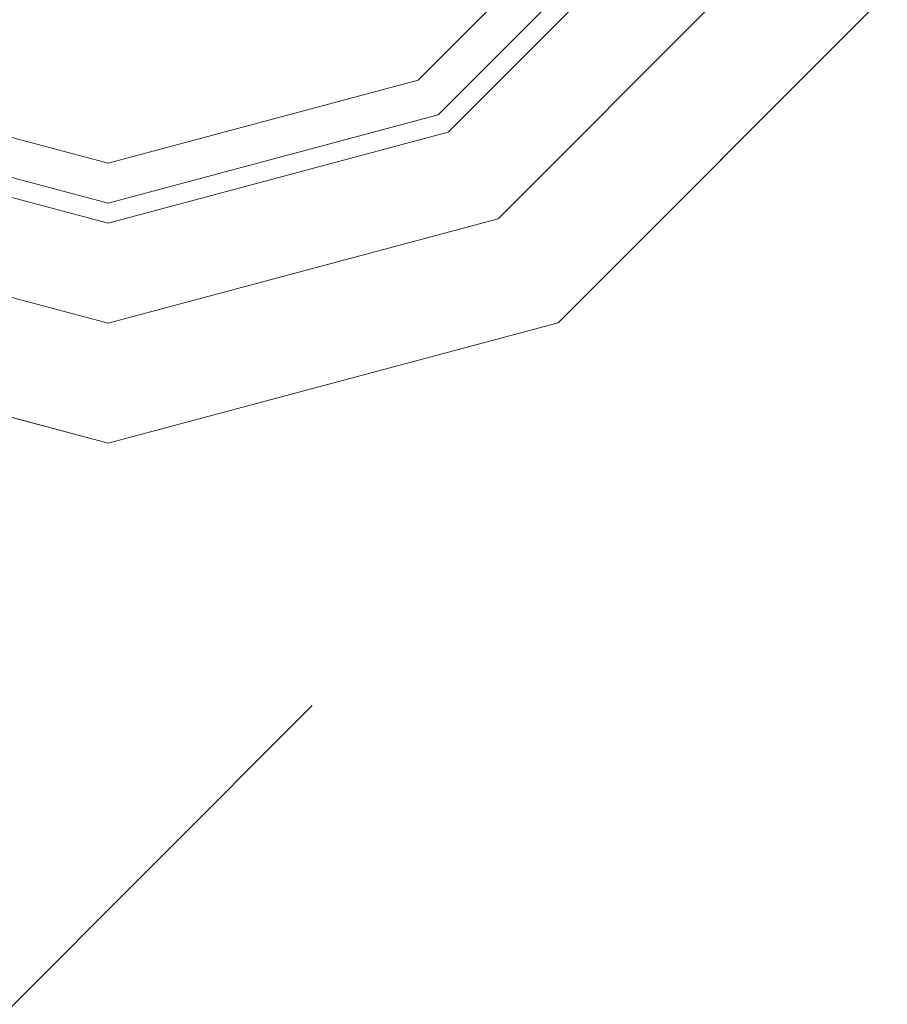
# Model space of a CAD drawing. Units: inches. Extents: x 375 to 1122, y 27 to 1069.
# Tile 53 of 155: x 725.537 to 730.88, y 308.183 to 314.242. Entities that reach past the tile are written whole.
import ezdxf

# ---------------------------------------------------------------- set-up
doc = ezdxf.new("R2010")
doc.units = ezdxf.units.IN
doc.layers.add('Furniture', color=30, linetype='Continuous', lineweight=18)

# ---------------------------------------------------------------- blocks, each defined once
blk = doc.blocks.new('A$C403C54AD')
blk.add_line((0.90685, 1.05977, -0.0006), (1.01943, 0.94723, -0.0006))
at = {"linetype": 'ByBlock'}
for points, invisible_edges in [([(0.81861, 1.08071, -0.03355), (0.84793, 1.09765, -0.02431), (0.79723, 1.14835, -0.02431), (0.7803, 1.11902, -0.03355)], 5), ([(0.84793, 1.09765, -0.0197), (0.83194, 1.08841, -0.0197), (0.78799, 1.13235, -0.0197), (0.79723, 1.14835, -0.0197)], 5), ([(0.83194, 1.08841, -0.0197), (0.81594, 1.07918, -0.02585), (0.77876, 1.11636, -0.02585), (0.78799, 1.13235, -0.0197)], 5), ([(0.81061, 1.0761, -0.04278), (0.81861, 1.08071, -0.03355), (0.7803, 1.11902, -0.03355), (0.77568, 1.11103, -0.04278)], 1), ([(0.81594, 1.07918, -0.02585), (0.72796, 1.02838, -0.02585), (0.72796, 1.02838, -0.02585), (0.77876, 1.11636, -0.02585)], 5), ([(0.83263, 1.02838, -0.03355), (0.86649, 1.02838, -0.02431), (0.84793, 1.09765, -0.02431), (0.81861, 1.08071, -0.03355)], 5), ([(0.86649, 1.02838, -0.0197), (0.84802, 1.02838, -0.0197), (0.83194, 1.08841, -0.0197), (0.84793, 1.09765, -0.0197)], 5), ([(0.84802, 1.02838, -0.0197), (0.82955, 1.02838, -0.02585), (0.81594, 1.07918, -0.02585), (0.83194, 1.08841, -0.0197)], 5), ([(0.82339, 1.02838, -0.04278), (0.83263, 1.02838, -0.03355), (0.81861, 1.08071, -0.03355), (0.81061, 1.0761, -0.04278)], 5), ([(0.82955, 1.02838, -0.02585), (0.72796, 1.02838, -0.02585), (0.72796, 1.02838, -0.02585), (0.81594, 1.07918, -0.02585)], 5), ([(0.81594, 0.97759, -0.02585), (0.72796, 1.02838, -0.02585), (0.72796, 1.02838, -0.02585), (0.82955, 1.02838, -0.02585)], 5), ([(0.77876, 0.94041, -0.02585), (0.72796, 1.02838, -0.02585), (0.72796, 1.02838, -0.02585), (0.81594, 0.97759, -0.02585)], 5), ([(0.81061, 0.98067, -0.04278), (0.81861, 0.97605, -0.03355), (0.83263, 1.02838, -0.03355), (0.82339, 1.02838, -0.04278)], 5), ([(0.83194, 0.96835, -0.0197), (0.81594, 0.97759, -0.02585), (0.82955, 1.02838, -0.02585), (0.84802, 1.02838, -0.0197)], 5), ([(0.81861, 0.97605, -0.03355), (0.84793, 0.95912, -0.02431), (0.86649, 1.02838, -0.02431), (0.83263, 1.02838, -0.03355)], 5), ([(0.84793, 0.95912, -0.0197), (0.83194, 0.96835, -0.0197), (0.84802, 1.02838, -0.0197), (0.86649, 1.02838, -0.0197)], 5)]:
    blk.add_3dface(points, dxfattribs=dict(at, invisible_edges=invisible_edges))
for points in [[(0.84793, 1.09765, -0.02431), (0.84793, 1.09765, -0.0197), (0.79723, 1.14835, -0.0197), (0.79723, 1.14835, -0.02431)], [(0.86649, 1.02838, -0.02431), (0.86649, 1.02838, -0.0197), (0.84793, 1.09765, -0.0197), (0.84793, 1.09765, -0.02431)], [(0.84793, 0.95912, -0.02431), (0.84793, 0.95912, -0.0197), (0.86649, 1.02838, -0.0197), (0.86649, 1.02838, -0.02431)]]:
    blk.add_3dface(points, dxfattribs=at)

msp = doc.modelspace()

# ---------------------------------------------------------------- block references
at = {"layer": 'Furniture', "xscale": 39.9918517141215, "yscale": 39.9918517141215, "zscale": 39.9918517141215, "rotation": 270}
msp.add_blockref('A$C403C54AD', (684.9549, 346.2875, 0.024), dxfattribs=at)

doc.saveas('drawing.dxf')
